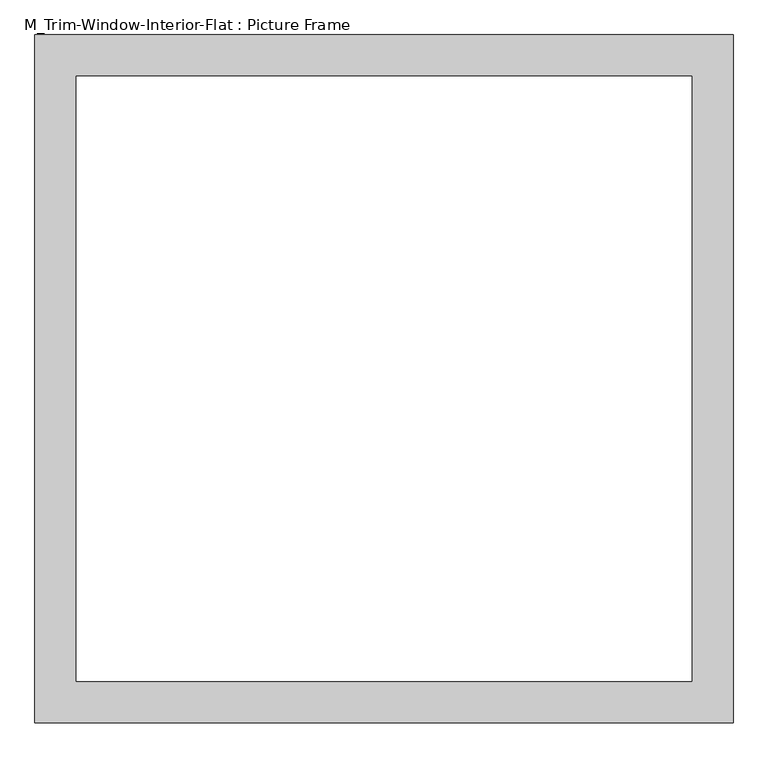
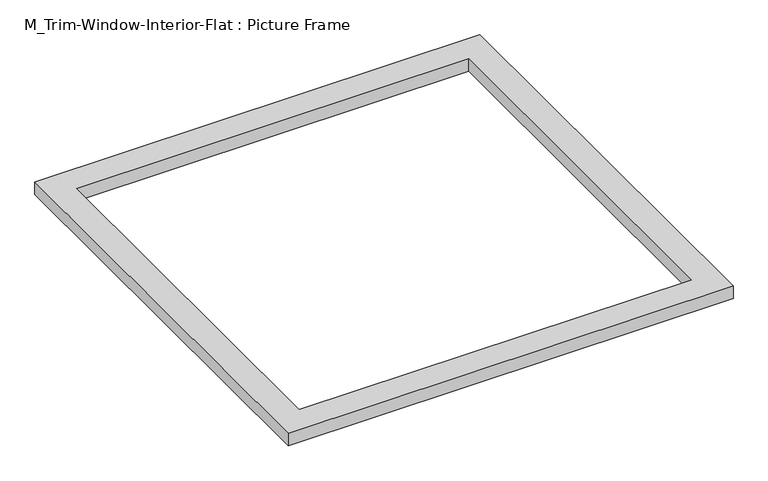
"""IFC4 building model written with IfcOpenShell, lengths in millimetres: proxy geometry, M_Trim-Window-Interior-Flat : Picture Frame."""

from ifc_helpers import new_model, si_unit, origin, origin_with_axes, place, context, project, spatial, polyline, outline, extrude, source, transform, mapped, element, save


def m_trim_window_interior_flat_picture_frame_b6dd03a6(model_context):
    return source(origin(), model_context, "Body", "SweptSolid", [
        extrude(outline(polyline([(504.5, 47.3), (504.5, -947.3), (-504.5, -947.3), (-504.5, 47.3), (504.5, 47.3)]), holes=[polyline([(444.5, -12.7), (-444.5, -12.7), (-444.5, -887.3), (444.5, -887.3), (444.5, -12.7)])]), origin_with_axes(), (0.0, 0.0, 1.0), 30.0),
    ])


if __name__ == "__main__":
    model = new_model("IFC4")
    model_context = context("Model", 3, world=origin())
    ifc_project = project(units=[si_unit("LENGTHUNIT", "METRE", prefix="MILLI")], contexts=[model_context])
    site = spatial("IfcSite", under=ifc_project)
    building = spatial("IfcBuilding", under=site)
    placement = place(None, origin())
    m_trim_window_interior_flat_picture_frame_shape = m_trim_window_interior_flat_picture_frame_b6dd03a6(model_context)
    element("IfcBuildingElementProxy", 1, Name="M_Trim-Window-Interior-Flat : Picture Frame", ObjectType="M_Trim-Window-Interior-Flat : Picture Frame", at=placement, inside=building, context=model_context, shape_type="MappedRepresentation", body=[
        mapped(m_trim_window_interior_flat_picture_frame_shape, transform((0.0, 0.0, 0.0), x_axis=(1.0, 0.0, 0.0), y_axis=(0.0, 1.0, 0.0), z_axis=(0.0, 0.0, 1.0))),
    ])
    save(model, "model.ifc")

# Revit data of these elements
# Type "M_Trim-Window-Interior-Flat : Picture Frame"
#   Trim Thickness_Picture Frame = 0' - 1.1811"
#   Trim Width = 0' - 2.3622"
#   Trim Thickness_with Sill = 0' - 0.7874"
#   Sill Thickness = 0' - 1.1811"
#   Opening Width [instance default] = 1' - 11.62205"
#   Opening Height [instance default] = 2' - 11.43307"
#   Default Elevation = 3' - 11.24409"
#   Sill = no
#   Picture Frame = yes
#   Trim Material [instance default] = none
# Element 1 (IfcBuildingElementProxy, "M_Trim-Window-Interior-Flat : Picture Frame")
#   Opening Width = 3' - 0"
#   Trim Material = Wood - Stained
#   Materials on its faces: "Wood - Stained"
# Materials
#   "Wood - Stained": class "Wood", colour RGB 224 178 126, transparency 0, Cost = 0
